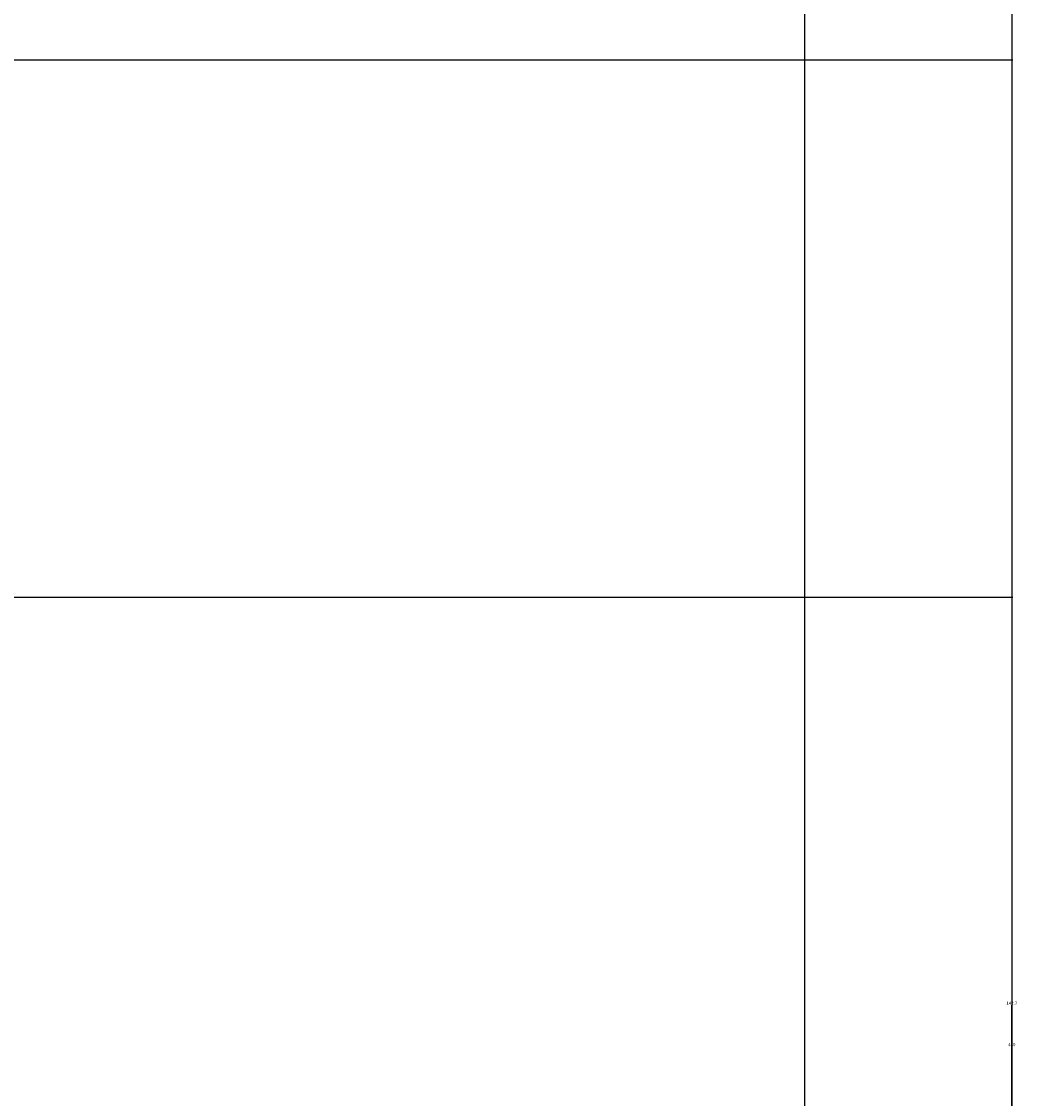
# Model space of a CAD drawing. Units: inches. Extents: x -26 to 776, y -22 to 650.
# Tile 59 of 62: x 601 to 776, y 226 to 415. Entities that reach past the tile are written whole.
import ezdxf

# ---------------------------------------------------------------- set-up
doc = ezdxf.new("R2010")
doc.units = ezdxf.units.IN
doc.header["$MEASUREMENT"] = 0
doc.layers.add('A-ANNO-DIMS', color=2, linetype='Continuous', lineweight=18)
doc.styles.get("Standard").update_dxf_attribs({"font": 'arial.ttf'})
doc.dimstyles.get("Standard").update_dxf_attribs({"dimtxt": 0.5625, "dimasz": 0.18, "dimexe": 0.18, "dimexo": 0.0625, "dimgap": 0.09, "dimtad": 0, "dimtih": 1, "dimtoh": 1, "dimdec": 4, "dimzin": 0, "dimdsep": 46, "dimlunit": 4, "dimtxsty": 'Standard', "dimcen": 0.09, "dimadec": 0, "dimazin": 0, "dimtfac": 1, "dimtdec": 4, "dimtofl": 0, "dimtmove": 0, "dimatfit": 3, "dimfxl": 1, "dimtolj": 1, "dimtzin": 0, "dimarcsym": 0})

# ---------------------------------------------------------------- blocks, each defined once
blk = doc.blocks.new('*D20')
at = {"layer": 'A-ANNO-DIMS', "color": 0, "lineweight": -2, "transparency": 16777216}
for p, q in [((425.81, 455.47), (775.34, 455.47)), ((775.16, 455.29), (775.16, 235.85)), ((775.16, 15.66), (775.16, 235.1)), ((425.81, 15.48), (775.34, 15.48))]:
    blk.add_line(p, q, dxfattribs=at)
at = {"layer": 'A-ANNO-DIMS', "color": 0, "transparency": 16777216}
for points in [[(775.13, 455.29), (775.19, 455.29), (775.16, 455.47)], [(775.13, 15.66), (775.19, 15.66), (775.16, 15.48)]]:
    blk.add_solid(points, dxfattribs=at)
at = {"layer": 'Defpoints', "color": 0, "transparency": 16777216}
for p in [(425.74, 455.47), (775.16, 455.47), (425.74, 15.48)]:
    blk.add_point(p, dxfattribs=at)
at = {"layer": 'A-ANNO-DIMS', "color": 0, "transparency": 16777216, "insert": (775.16, 235.48), "char_height": 0.562, "attachment_point": 5}
blk.add_mtext('\\A1;440', dxfattribs=at)
blk = doc.blocks.new('*D28')
at = {"layer": 'A-ANNO-DIMS', "color": 0, "lineweight": -2, "transparency": 16777216}
for p, q in [((285.08, 314.12), (775.34, 314.12)), ((775.16, 313.94), (775.16, 243.14)), ((775.16, 171.6), (775.16, 242.4)), ((285.08, 171.42), (775.34, 171.42))]:
    blk.add_line(p, q, dxfattribs=at)
at = {"layer": 'A-ANNO-DIMS', "color": 0, "transparency": 16777216}
for points in [[(775.13, 313.94), (775.19, 313.94), (775.16, 314.12)], [(775.13, 171.6), (775.19, 171.6), (775.16, 171.42)]]:
    blk.add_solid(points, dxfattribs=at)
at = {"layer": 'Defpoints', "color": 0, "transparency": 16777216}
for p in [(285.02, 314.12), (775.16, 314.12), (285.02, 171.42)]:
    blk.add_point(p, dxfattribs=at)
at = {"layer": 'A-ANNO-DIMS', "color": 0, "transparency": 16777216, "insert": (775.16, 242.77), "char_height": 0.562, "attachment_point": 5}
blk.add_mtext('\\A1;142.7', dxfattribs=at)
blk = doc.blocks.new('*D45')
at = {"layer": 'A-ANNO-DIMS', "color": 0, "lineweight": -2, "transparency": 16777216}
for p, q in [((507.74, 408.64), (775.34, 408.64)), ((775.16, 408.46), (775.16, 212.44)), ((775.16, 15.66), (775.16, 211.68)), ((586, 15.48), (775.34, 15.48))]:
    blk.add_line(p, q, dxfattribs=at)
at = {"layer": 'A-ANNO-DIMS', "color": 0, "transparency": 16777216}
for points in [[(775.13, 408.46), (775.19, 408.46), (775.16, 408.64)], [(775.13, 15.66), (775.19, 15.66), (775.16, 15.48)]]:
    blk.add_solid(points, dxfattribs=at)
at = {"layer": 'Defpoints', "color": 0, "transparency": 16777216}
for p in [(507.68, 408.64), (775.16, 408.64), (585.94, 15.48)]:
    blk.add_point(p, dxfattribs=at)
at = {"layer": 'A-ANNO-DIMS', "color": 0, "transparency": 16777216, "insert": (775.16, 212.06), "char_height": 0.562, "attachment_point": 5}
blk.add_mtext('\\A1;393.16', dxfattribs=at)
blk = doc.blocks.new('*D48')
at = {"layer": 'A-ANNO-DIMS', "color": 0, "lineweight": -2, "transparency": 16777216}
for p, q in [((545.03, 67.41), (545.03, 649.86)), ((545.21, 649.68), (640.88, 649.68)), ((738.57, 649.68), (642.9, 649.68)), ((738.75, 50.91), (738.75, 649.86))]:
    blk.add_line(p, q, dxfattribs=at)
at = {"layer": 'A-ANNO-DIMS', "color": 0, "transparency": 16777216}
for points in [[(545.21, 649.71), (545.21, 649.65), (545.03, 649.68)], [(738.57, 649.71), (738.57, 649.65), (738.75, 649.68)]]:
    blk.add_solid(points, dxfattribs=at)
at = {"layer": 'Defpoints', "color": 0, "transparency": 16777216}
for p in [(738.75, 649.68), (545.03, 67.35), (738.75, 50.85)]:
    blk.add_point(p, dxfattribs=at)
at = {"layer": 'A-ANNO-DIMS', "color": 0, "transparency": 16777216, "insert": (641.89, 649.68), "char_height": 0.562, "attachment_point": 5}
blk.add_mtext('\\A1;193.7', dxfattribs=at)

msp = doc.modelspace()

# ---------------------------------------------------------------- dimensions: what is measured, and where the dimension line sits
at = {"layer": 'A-ANNO-DIMS'}
dim = msp.add_linear_dim(base=(738.7503, 649.6763), p1=(545.0331, 67.3523), p2=(738.7503, 50.8482), dimstyle='Standard', override={"dimdec": 1, "dimlfac": 1, "dimrnd": 0, "dimzin": 0, "dimdsep": 46, "dimlunit": 2}, dxfattribs=at)
dim.commit()
dim.dimension.update_dxf_attribs({"geometry": '*D48', "text_midpoint": (641.8917, 649.6763)})
for base, p1, p2, override, picture, middle in [((775.1553, 455.4717), (425.7434, 15.4824), (425.7434, 455.4717), {"dimdec": 0, "dimlfac": 1, "dimrnd": 0, "dimzin": 0, "dimdsep": 46, "dimlunit": 2}, '*D20', (775.1553, 235.477)), ((775.1553, 408.6389), (585.9354, 15.4824), (507.6759, 408.6389), {"dimdec": 2, "dimlfac": 1, "dimrnd": 0, "dimzin": 0, "dimdsep": 46, "dimlunit": 2}, '*D45', (775.1553, 212.0606)), ((775.1553, 314.119), (285.0179, 171.4173), (285.0179, 314.119), {"dimdec": 1, "dimlfac": 1, "dimrnd": 0, "dimzin": 0, "dimdsep": 46, "dimlunit": 2}, '*D28', (775.1553, 242.7682))]:
    dim = msp.add_linear_dim(base=base, p1=p1, p2=p2, angle=90, dimstyle='Standard', override=override, dxfattribs=at)
    dim.commit()
    dim.dimension.update_dxf_attribs({"geometry": picture, "text_midpoint": middle})

doc.saveas('drawing.dxf')
